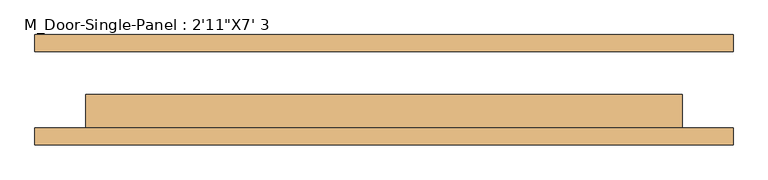
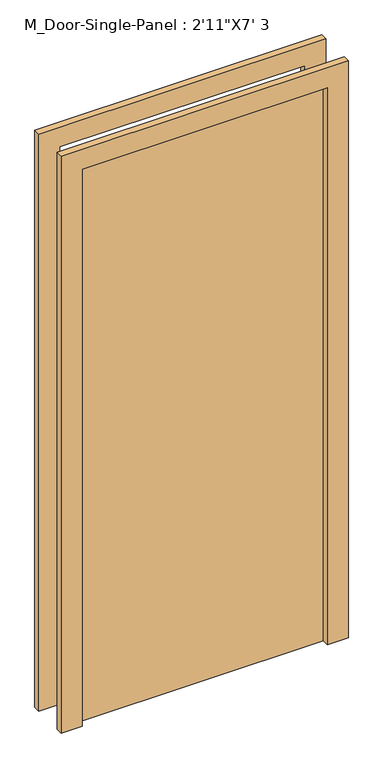
"""IFC4 building model written with IfcOpenShell, lengths in millimetres: door geometry."""

from ifc_helpers import new_model, si_unit, frame, origin, origin_with_axes, place, context, project, spatial, polyline, outline, extrude, source, transform, mapped, element, save


def door_1991e9a2(model_context):
    return source(origin(), model_context, "Body", "SweptSolid", [
        extrude(outline(polyline([(444.5, -7.15), (444.5, -57.15), (-444.5, -57.15), (-444.5, -7.15), (444.5, -7.15)])), origin_with_axes(), (0.0, 0.0, 1.0), 2133.6),
        extrude(outline(polyline([(2209.8, 520.7), (2209.8, -520.7), (0.0, -520.7), (0.0, -444.5), (2133.6, -444.5), (2133.6, 444.5), (0.0, 444.5), (0.0, 520.7), (2209.8, 520.7)])), frame((0.0, 57.15, 0.0), z_axis=(0.0, 1.0, 0.0), x_axis=(0.0, 0.0, 1.0)), (0.0, 0.0, 1.0), 25.0),
        extrude(outline(polyline([(2209.8, -520.7), (0.0, -520.7), (0.0, -444.5), (2133.6, -444.5), (2133.6, 444.5), (0.0, 444.5), (0.0, 520.7), (2209.8, 520.7), (2209.8, -520.7)])), frame((0.0, -82.15, 0.0), z_axis=(0.0, 1.0, 0.0), x_axis=(0.0, 0.0, 1.0)), (0.0, 0.0, 1.0), 25.0),
    ])


if __name__ == "__main__":
    model = new_model("IFC4")
    model_context = context("Model", 3, world=origin())
    ifc_project = project(units=[si_unit("LENGTHUNIT", "METRE", prefix="MILLI")], contexts=[model_context])
    site = spatial("IfcSite", under=ifc_project)
    building = spatial("IfcBuilding", under=site)
    placement = place(None, origin())
    door_shape = door_1991e9a2(model_context)
    element("IfcDoor", 1, ObjectType="M_Door-Single-Panel : 2'11\"X7' 3", at=placement, inside=building, context=model_context, shape_type="MappedRepresentation", body=[
        mapped(door_shape, transform((0.0, 0.0, 0.0), x_axis=(1.0, 0.0, 0.0), y_axis=(0.0, 1.0, 0.0), z_axis=(0.0, 0.0, 1.0))),
    ])
    save(model, "model.ifc")

# Revit data of these elements
# Type "M_Door-Single-Panel : 2'11\"X7' 3"
#   Type Mark = "12"
#   Construction Type Id = "DOOR"
#   Assembly Code = "C1020300"
#   Analytic Construction = "Wooden"
#   Thickness = 0' - 1.9685"
#   Thermal Resistance (R) = 2.5876 (h·ft²·°F)/BTU
#   Swing Angle [instance default] = 90.00°
#   Heat Transfer Coefficient (U) = 0.3865 BTU/(h·ft²·°F)
#   Height = 7' - 0"
#   Trim Projection Ext = 0' - 0.98425"
#   Trim Projection Int = 0' - 0.98425"
#   Trim Width = 0' - 3.14961"
#   Width = 2' - 11"
#   Define Thermal Properties by = 1
#   Panel Material = Wood - Birch - Solid Stained Light Low Gloss
#   Trim Material = Paint - Sienna
#   Visual Light Transmittance = 0
#   Solar Heat Gain Coefficient = 0
#   Function = (empty or 0)
#   Wall Closure = (empty or 0)
# Element 1 (IfcDoor, "M_Door-Single-Panel : 2'11\"X7' 3")
#   Materials on its faces: "Paint - Sienna", "Wood - Birch - Solid Stained Light Low Gloss"
# Materials
#   "Wood - Birch - Solid Stained Light Low Gloss": class "Wood", colour RGB 210 159 95, transparency 0, Cost = 0
#   "Paint - Sienna": colour RGB 118 70 51, transparency 0, Cost = 0
